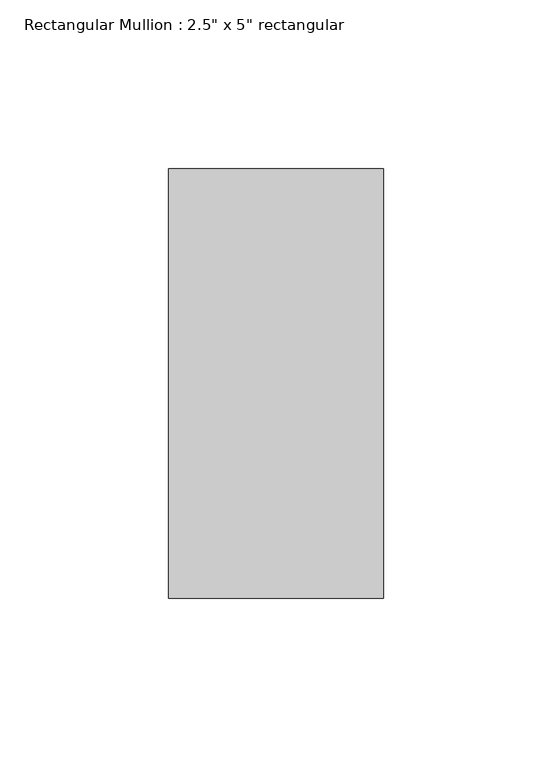
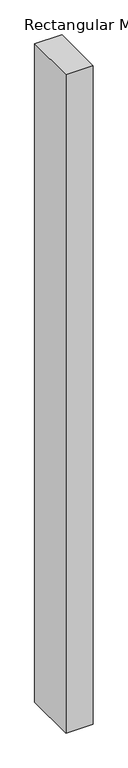
"""IFC4 building model written with IfcOpenShell, lengths in millimetres: member geometry."""

from ifc_helpers import new_model, si_unit, frame, origin, place, context, project, spatial, polyline, outline, extrude, source, transform, mapped, element, save


def member_1ecbbc04(model_context):
    return source(origin(), model_context, "Body", "SweptSolid", [
        extrude(outline(polyline([(31.75, 63.5), (31.75, -63.5), (-31.75, -63.5), (-31.75, 63.5), (31.75, 63.5)])), frame((0.0, 0.0, -1630.7489674), z_axis=(0.0, 0.0, 1.0), x_axis=(1.0, 0.0, 0.0)), (0.0, 0.0, 1.0), 1630.7489674),
    ])


if __name__ == "__main__":
    model = new_model("IFC4")
    model_context = context("Model", 3, world=origin())
    ifc_project = project(units=[si_unit("LENGTHUNIT", "METRE", prefix="MILLI")], contexts=[model_context])
    site = spatial("IfcSite", under=ifc_project)
    building = spatial("IfcBuilding", under=site)
    placement = place(None, origin())
    member_shape = member_1ecbbc04(model_context)
    element("IfcMember", 1, ObjectType="Rectangular Mullion : 2.5\" x 5\" rectangular", at=placement, inside=building, context=model_context, shape_type="MappedRepresentation", body=[
        mapped(member_shape, transform((0.0, 0.0, 0.0), x_axis=(1.0, 0.0, 0.0), y_axis=(0.0, 1.0, 0.0), z_axis=(0.0, 0.0, 1.0))),
    ])
    save(model, "model.ifc")

# Revit data of these elements
# Type "Rectangular Mullion : 2.5\" x 5\" rectangular"
#   built-in parameter 1007304 = 0.416667 (stored number, unit not read)
#   built-in parameter 1007301 = 0.104167 (stored number, unit not read)
#   built-in parameter 1007300 = 0.104167 (stored number, unit not read)
# Element 1 (IfcMember, "Rectangular Mullion : 2.5\" x 5\" rectangular")
#   Materials on its faces: "Aluminum"
# Materials
#   "Aluminum": class "Metal", colour RGB 247 247 247, transparency 0, Description = "Aluminum 6061", Cost = 0
